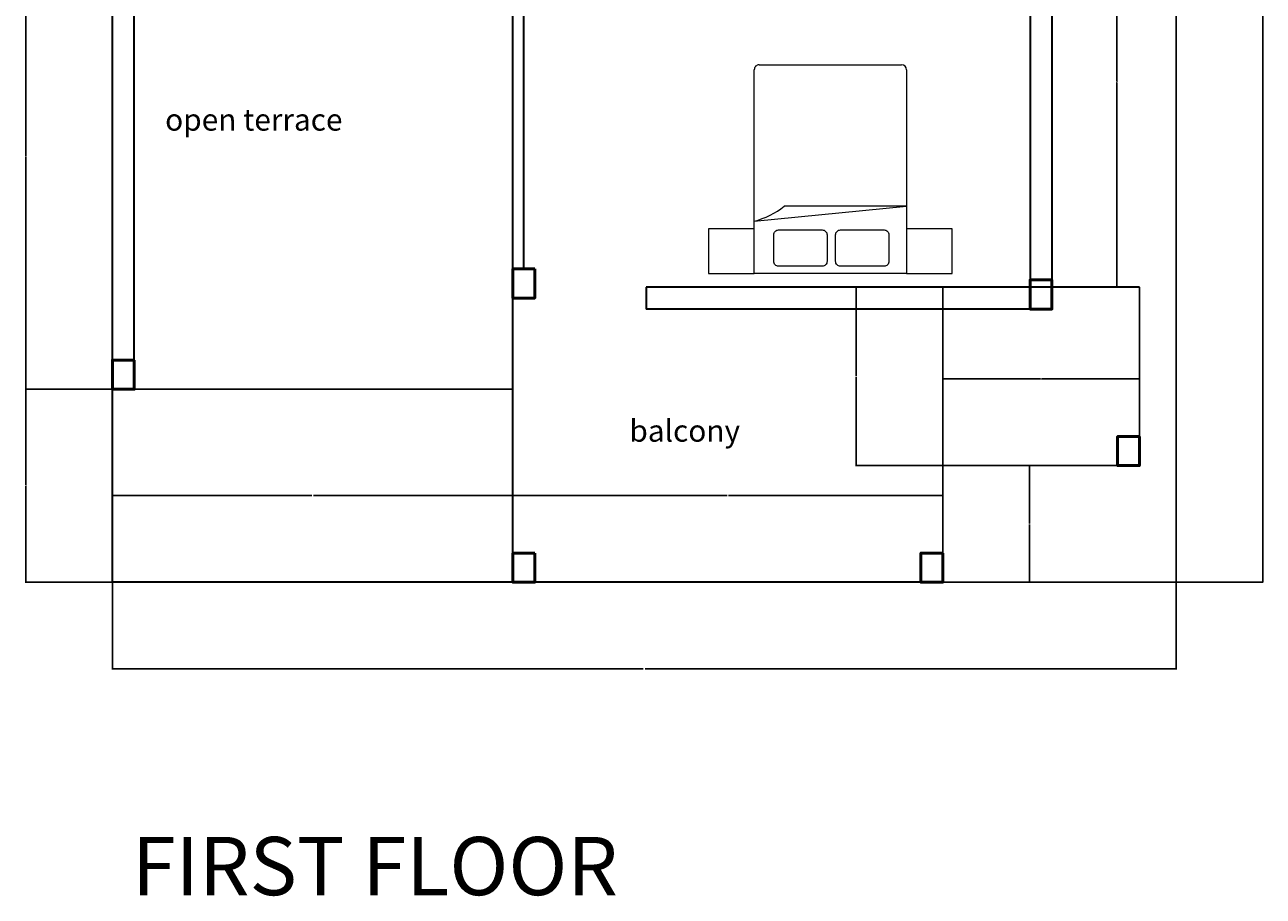
# Model space of a CAD drawing. Units: inches. Extents: x 1748 to 3019, y 1454 to 2188.
# Tile 3 of 4: x 2509 to 3019, y 1459 to 1818. Entities that reach past the tile are written whole.
import ezdxf

# ---------------------------------------------------------------- set-up
doc = ezdxf.new("R2010")
doc.units = ezdxf.units.IN
for name, color, linetype, lineweight in [('A-ANNO-DIMS', 2, 'Continuous', 18), ('A-ANNO-TEXT', 7, 'Continuous', 35), ('A-AREA-IDEN', 134, 'Continuous', 18), ('A-COLS', 120, 'Continuous', 50), ('A-FLOR', 8, 'Continuous', 25), ('A-WALL', 7, 'Continuous', 35), ('bed', 21, 'Continuous', 18)]:
    doc.layers.add(name, color=color, linetype=linetype, lineweight=lineweight)
doc.styles.get("Standard").update_dxf_attribs({"font": 'arial.ttf'})
doc.dimstyles.get("Standard").update_dxf_attribs({"dimtxt": 0.18, "dimasz": 0.18, "dimexe": 0.18, "dimexo": 0.0625, "dimgap": 0.09, "dimtad": 0, "dimtih": 1, "dimtoh": 1, "dimdec": 4, "dimzin": 0, "dimdsep": 46, "dimtxsty": 'Standard', "dimcen": 0.09, "dimadec": 0, "dimazin": 0, "dimtfac": 1, "dimtdec": 4, "dimtofl": 0, "dimtmove": 0, "dimatfit": 3, "dimfxl": 1, "dimtolj": 1, "dimtzin": 0, "dimarcsym": 0})

# ---------------------------------------------------------------- blocks, each defined once
blk = doc.blocks.new('BED-DOUBLE-NIGHTSTANDS')
for p, q in [((0, 81.51), (83.98, 81.51)), ((0, 18.79), (0, 81.51)), ((21.61, 81.51), (27.83, 18.79)), ((85.98, 79.51), (85.98, 20.79)), ((27.83, 18.79), (27.83, 69.19)), ((83.98, 18.79), (0, 18.79))]:
    blk.add_line(p, q)
for points in [[(0, 81.51), (18.52, 81.51), (18.52, 100.3), (0, 100.3)], [(0, 0), (18.52, 0), (18.52, 18.79), (0, 18.79)]]:
    blk.add_lwpolyline(points, close=True)
for points in [[(5.06, 73.49), (16.01, 73.49, -0.414214), (18.01, 71.49), (18.01, 53.51, -0.414214), (16.01, 51.51), (5.06, 51.51, -0.414214), (3.06, 53.51), (3.06, 71.49, -0.414214)], [(5.06, 47.99), (16.01, 47.99, -0.414214), (18.01, 45.99), (18.01, 28.02, -0.414214), (16.01, 26.02), (5.06, 26.02, -0.414214), (3.06, 28.02), (3.06, 45.99, -0.414214)]]:
    blk.add_lwpolyline(points, format="xyb", close=True)
for centre, radius, start, end in [((52.42, 89.31), 31.78, 194.1991, 219.2902), ((83.98, 79.51), 2, 0, 90), ((83.98, 79.51), 2, 0, 90), ((83.98, 20.79), 2, 270, 0)]:
    blk.add_arc(centre, radius, start, end)
blk = doc.blocks.new('COLUMN-9X12')
blk.add_lwpolyline([(9, 12), (9, 0), (0, 0), (0, 12)], close=True)
blk = doc.blocks.new('*D44')
at = {"layer": 'A-ANNO-DIMS', "color": 0, "lineweight": -2, "transparency": 16777216}
for p, q in [((2982.74, 1877), (2982.74, 1552.06)), ((2544.64, 1587.88), (2544.64, 1552.06)), ((2544.82, 1552.24), (2763.31, 1552.24)), ((2982.56, 1552.24), (2764.07, 1552.24))]:
    blk.add_line(p, q, dxfattribs=at)
at = {"layer": 'A-ANNO-DIMS', "color": 0, "transparency": 16777216}
for points in [[(2544.82, 1552.27), (2544.82, 1552.21), (2544.64, 1552.24)], [(2982.56, 1552.27), (2982.56, 1552.21), (2982.74, 1552.24)]]:
    blk.add_solid(points, dxfattribs=at)
at = {"layer": 'Defpoints', "color": 0, "transparency": 16777216}
for p in [(2982.74, 1877.06), (2544.64, 1587.94), (2982.74, 1552.24)]:
    blk.add_point(p, dxfattribs=at)
at = {"layer": 'A-ANNO-DIMS', "color": 0, "transparency": 16777216, "insert": (2763.69, 1552.24), "char_height": 0.18, "attachment_point": 5}
blk.add_mtext('\\A1;438.1', dxfattribs=at)
blk = doc.blocks.new('*D45')
at = {"layer": 'A-ANNO-DIMS', "color": 0, "lineweight": -2, "transparency": 16777216}
for p, q in [((2931.7, 2151.94), (3018.62, 2151.94)), ((3018.44, 2151.76), (3018.44, 1870.12)), ((3018.44, 1588.12), (3018.44, 1869.76)), ((2886.7, 1587.94), (3018.62, 1587.94))]:
    blk.add_line(p, q, dxfattribs=at)
at = {"layer": 'A-ANNO-DIMS', "color": 0, "transparency": 16777216}
for points in [[(3018.41, 2151.76), (3018.47, 2151.76), (3018.44, 2151.94)], [(3018.41, 1588.12), (3018.47, 1588.12), (3018.44, 1587.94)]]:
    blk.add_solid(points, dxfattribs=at)
at = {"layer": 'Defpoints', "color": 0, "transparency": 16777216}
for p in [(2931.64, 2151.94), (3018.44, 2151.94), (2886.64, 1587.94)]:
    blk.add_point(p, dxfattribs=at)
at = {"layer": 'A-ANNO-DIMS', "color": 0, "transparency": 16777216, "insert": (3018.44, 1869.94), "char_height": 0.18, "attachment_point": 5}
blk.add_mtext('\\A1;564', dxfattribs=at)
blk = doc.blocks.new('*D53')
at = {"layer": 'A-ANNO-DIMS', "color": 0, "lineweight": -2, "transparency": 16777216}
for p, q in [((2544.57, 1859.39), (2508.76, 1859.39)), ((2508.94, 1859.21), (2508.94, 1763.6)), ((2508.94, 1667.62), (2508.94, 1763.23)), ((2544.57, 1667.44), (2508.76, 1667.44))]:
    blk.add_line(p, q, dxfattribs=at)
at = {"layer": 'A-ANNO-DIMS', "color": 0, "transparency": 16777216}
for points in [[(2508.91, 1859.21), (2508.97, 1859.21), (2508.94, 1859.39)], [(2508.91, 1667.62), (2508.97, 1667.62), (2508.94, 1667.44)]]:
    blk.add_solid(points, dxfattribs=at)
at = {"layer": 'Defpoints', "color": 0, "transparency": 16777216}
for p in [(2508.94, 1859.39), (2544.64, 1859.39), (2544.64, 1667.44)]:
    blk.add_point(p, dxfattribs=at)
at = {"layer": 'A-ANNO-DIMS', "color": 0, "transparency": 16777216, "insert": (2508.94, 1763.42), "char_height": 0.18, "attachment_point": 5}
blk.add_mtext('\\A1;191.95', dxfattribs=at)
blk = doc.blocks.new('*D54')
at = {"layer": 'A-ANNO-DIMS', "color": 0, "lineweight": -2, "transparency": 16777216}
for p, q in [((2544.57, 1667.44), (2508.76, 1667.44)), ((2508.94, 1667.26), (2508.94, 1627.87)), ((2508.94, 1588.12), (2508.94, 1627.51)), ((2544.57, 1587.94), (2508.76, 1587.94))]:
    blk.add_line(p, q, dxfattribs=at)
at = {"layer": 'A-ANNO-DIMS', "color": 0, "transparency": 16777216}
for points in [[(2508.91, 1667.26), (2508.97, 1667.26), (2508.94, 1667.44)], [(2508.91, 1588.12), (2508.97, 1588.12), (2508.94, 1587.94)]]:
    blk.add_solid(points, dxfattribs=at)
at = {"layer": 'Defpoints', "color": 0, "transparency": 16777216}
for p in [(2508.94, 1667.44), (2544.64, 1667.44), (2544.64, 1587.94)]:
    blk.add_point(p, dxfattribs=at)
at = {"layer": 'A-ANNO-DIMS', "color": 0, "transparency": 16777216, "insert": (2508.94, 1627.69), "char_height": 0.18, "attachment_point": 5}
blk.add_mtext('\\A1;79.5', dxfattribs=at)
blk = doc.blocks.new('*D55')
at = {"layer": 'A-ANNO-DIMS', "color": 0, "lineweight": -2, "transparency": 16777216}
for p, q in [((2922.7, 1878.41), (2958.52, 1878.41)), ((2958.34, 1878.23), (2958.34, 1794.11)), ((2958.34, 1709.62), (2958.34, 1793.74)), ((2922.7, 1709.44), (2958.52, 1709.44))]:
    blk.add_line(p, q, dxfattribs=at)
at = {"layer": 'A-ANNO-DIMS', "color": 0, "transparency": 16777216}
for points in [[(2958.31, 1878.23), (2958.37, 1878.23), (2958.34, 1878.41)], [(2958.31, 1709.62), (2958.37, 1709.62), (2958.34, 1709.44)]]:
    blk.add_solid(points, dxfattribs=at)
at = {"layer": 'Defpoints', "color": 0, "transparency": 16777216}
for p in [(2922.64, 1878.41), (2922.64, 1709.44), (2958.34, 1709.44)]:
    blk.add_point(p, dxfattribs=at)
at = {"layer": 'A-ANNO-DIMS', "color": 0, "transparency": 16777216, "insert": (2958.34, 1793.93), "char_height": 0.18, "attachment_point": 5}
blk.add_mtext('\\A1;168.97', dxfattribs=at)
blk = doc.blocks.new('*D56')
at = {"layer": 'A-ANNO-DIMS', "color": 0, "lineweight": -2, "transparency": 16777216}
for p, q in [((2544.64, 1588), (2544.64, 1623.82)), ((2544.82, 1623.64), (2626.85, 1623.64)), ((2709.46, 1623.64), (2627.42, 1623.64)), ((2709.64, 1588), (2709.64, 1623.82))]:
    blk.add_line(p, q, dxfattribs=at)
at = {"layer": 'A-ANNO-DIMS', "color": 0, "transparency": 16777216}
for points in [[(2544.82, 1623.67), (2544.82, 1623.61), (2544.64, 1623.64)], [(2709.46, 1623.67), (2709.46, 1623.61), (2709.64, 1623.64)]]:
    blk.add_solid(points, dxfattribs=at)
at = {"layer": 'Defpoints', "color": 0, "transparency": 16777216}
for p in [(2709.64, 1623.64), (2544.64, 1587.94), (2709.64, 1587.94)]:
    blk.add_point(p, dxfattribs=at)
at = {"layer": 'A-ANNO-DIMS', "color": 0, "transparency": 16777216, "insert": (2627.14, 1623.64), "char_height": 0.18, "attachment_point": 5}
blk.add_mtext('\\A1;165', dxfattribs=at)
blk = doc.blocks.new('*D57')
at = {"layer": 'A-ANNO-DIMS', "color": 0, "lineweight": -2, "transparency": 16777216}
for p, q in [((2709.64, 1588), (2709.64, 1623.82)), ((2709.82, 1623.64), (2797.85, 1623.64)), ((2886.46, 1623.64), (2798.42, 1623.64)), ((2886.64, 1588), (2886.64, 1623.82))]:
    blk.add_line(p, q, dxfattribs=at)
at = {"layer": 'A-ANNO-DIMS', "color": 0, "transparency": 16777216}
for points in [[(2709.82, 1623.67), (2709.82, 1623.61), (2709.64, 1623.64)], [(2886.46, 1623.67), (2886.46, 1623.61), (2886.64, 1623.64)]]:
    blk.add_solid(points, dxfattribs=at)
at = {"layer": 'Defpoints', "color": 0, "transparency": 16777216}
for p in [(2886.64, 1623.64), (2709.64, 1587.94), (2886.64, 1587.94)]:
    blk.add_point(p, dxfattribs=at)
at = {"layer": 'A-ANNO-DIMS', "color": 0, "transparency": 16777216, "insert": (2798.14, 1623.64), "char_height": 0.18, "attachment_point": 5}
blk.add_mtext('\\A1;177', dxfattribs=at)
blk = doc.blocks.new('*D58')
at = {"layer": 'A-ANNO-DIMS', "color": 0, "lineweight": -2, "transparency": 16777216}
for p, q in [((2886.57, 1709.44), (2850.76, 1709.44)), ((2850.94, 1709.26), (2850.94, 1672.87)), ((2850.94, 1636.12), (2850.94, 1672.51)), ((2886.57, 1635.94), (2850.76, 1635.94))]:
    blk.add_line(p, q, dxfattribs=at)
at = {"layer": 'A-ANNO-DIMS', "color": 0, "transparency": 16777216}
for points in [[(2850.91, 1709.26), (2850.97, 1709.26), (2850.94, 1709.44)], [(2850.91, 1636.12), (2850.97, 1636.12), (2850.94, 1635.94)]]:
    blk.add_solid(points, dxfattribs=at)
at = {"layer": 'Defpoints', "color": 0, "transparency": 16777216}
for p in [(2850.94, 1709.44), (2886.64, 1709.44), (2886.64, 1635.94)]:
    blk.add_point(p, dxfattribs=at)
at = {"layer": 'A-ANNO-DIMS', "color": 0, "transparency": 16777216, "insert": (2850.94, 1672.69), "char_height": 0.18, "attachment_point": 5}
blk.add_mtext('\\A1;73.5', dxfattribs=at)
blk = doc.blocks.new('*D59')
at = {"layer": 'A-ANNO-DIMS', "color": 0, "lineweight": -2, "transparency": 16777216}
for p, q in [((2886.7, 1635.94), (2922.52, 1635.94)), ((2922.34, 1635.76), (2922.34, 1612.12)), ((2922.34, 1588.12), (2922.34, 1611.76)), ((2886.7, 1587.94), (2922.52, 1587.94))]:
    blk.add_line(p, q, dxfattribs=at)
at = {"layer": 'A-ANNO-DIMS', "color": 0, "transparency": 16777216}
for points in [[(2922.31, 1635.76), (2922.37, 1635.76), (2922.34, 1635.94)], [(2922.31, 1588.12), (2922.37, 1588.12), (2922.34, 1587.94)]]:
    blk.add_solid(points, dxfattribs=at)
at = {"layer": 'Defpoints', "color": 0, "transparency": 16777216}
for p in [(2886.64, 1635.94), (2886.64, 1587.94), (2922.34, 1587.94)]:
    blk.add_point(p, dxfattribs=at)
at = {"layer": 'A-ANNO-DIMS', "color": 0, "transparency": 16777216, "insert": (2922.34, 1611.94), "char_height": 0.18, "attachment_point": 5}
blk.add_mtext('\\A1;48', dxfattribs=at)
blk = doc.blocks.new('*D60')
at = {"layer": 'A-ANNO-DIMS', "color": 0, "lineweight": -2, "transparency": 16777216}
for p, q in [((2886.64, 1636), (2886.64, 1671.82)), ((2886.82, 1671.64), (2926.93, 1671.64)), ((2967.46, 1671.64), (2927.34, 1671.64)), ((2967.64, 1636), (2967.64, 1671.82))]:
    blk.add_line(p, q, dxfattribs=at)
at = {"layer": 'A-ANNO-DIMS', "color": 0, "transparency": 16777216}
for points in [[(2886.82, 1671.67), (2886.82, 1671.61), (2886.64, 1671.64)], [(2967.46, 1671.67), (2967.46, 1671.61), (2967.64, 1671.64)]]:
    blk.add_solid(points, dxfattribs=at)
at = {"layer": 'Defpoints', "color": 0, "transparency": 16777216}
for p in [(2967.64, 1671.64), (2886.64, 1635.94), (2967.64, 1635.94)]:
    blk.add_point(p, dxfattribs=at)
at = {"layer": 'A-ANNO-DIMS', "color": 0, "transparency": 16777216, "insert": (2927.14, 1671.64), "char_height": 0.18, "attachment_point": 5}
blk.add_mtext('\\A1;81', dxfattribs=at)

msp = doc.modelspace()

# ---------------------------------------------------------------- linework, layer by layer
at = {"layer": 'A-FLOR'}
for p, q in [((2886.6353, 1644.94), (2886.6353, 1709.44)), ((2967.6353, 1635.94), (2967.6353, 1709.44)), ((2544.6353, 1667.44), (2709.6353, 1667.44)), ((2958.6353, 1644.94), (2958.6353, 1647.94)), ((2886.6353, 1587.94), (2886.6353, 1644.94)), ((2967.6353, 1635.94), (2886.6353, 1635.94))]:
    msp.add_line(p, q, dxfattribs=at)
at = {"layer": 'A-WALL'}
for p, q in [((2922.6353, 2142.94), (2922.6353, 1709.44)), ((2714.1353, 1716.94), (2714.1353, 1863.94)), ((2553.6353, 1667.44), (2553.6353, 1859.44)), ((2709.6353, 1587.94), (2709.6353, 1859.44)), ((2967.6353, 1709.44), (2764.5076, 1709.44)), ((2764.5076, 1709.44), (2764.5076, 1700.44)), ((2931.6353, 1700.44), (2764.5076, 1700.44))]:
    msp.add_line(p, q, dxfattribs=at)
msp.add_lwpolyline([(2886.6353, 1587.94), (2544.6353, 1587.94), (2544.6353, 2151.94), (2931.6353, 2151.94), (2931.6353, 1709.44)], dxfattribs=at)

# ---------------------------------------------------------------- block references
at = {"layer": 'A-COLS'}
for p in [(2709.6349, 1704.94), (2922.6349, 1700.44), (2544.6349, 1667.44), (2958.6349, 1635.94), (2709.6349, 1587.94), (2877.6349, 1587.94)]:
    msp.add_blockref('COLUMN-9X12', p, dxfattribs=at)
at = {"layer": 'bed', "rotation": 89.99999999999962}
msp.add_blockref('BED-DOUBLE-NIGHTSTANDS', (2890.5185, 1715.017), dxfattribs=at)

# ---------------------------------------------------------------- texts
at = {"layer": 'A-ANNO-TEXT', "insert": (2552.6888, 1483.0463), "char_height": 24, "attachment_point": 1}
msp.add_mtext_dynamic_manual_height_columns('FIRST FLOOR', width=613.135788, gutter_width=12.5, heights=[0], dxfattribs=at)
at = {"layer": 'A-AREA-IDEN', "char_height": 9, "attachment_point": 1}
for s, width, insert in [('open terrace', 94.454348, (2566.381, 1782.9213)), ('balcony', 119.179894, (2757.5913, 1654.8119))]:
    msp.add_mtext_dynamic_manual_height_columns(s, width=width, gutter_width=12.5, heights=[0], dxfattribs=dict(at, insert=insert))

# ---------------------------------------------------------------- dimensions: what is measured, and where the dimension line sits
at = {"layer": 'A-ANNO-DIMS'}
for base, p1, p2, angle, override, picture, middle in [((3018.4428, 2151.94), (2886.6353, 1587.94), (2931.6353, 2151.94), 90, {"dimdec": 0, "dimlfac": 1, "dimrnd": 0, "dimzin": 0, "dimdsep": 46, "dimlunit": 2}, '*D45', (3018.4428, 1869.94)), ((2958.3353, 1709.44), (2922.6353, 1878.412), (2922.6353, 1709.44), 270, {"dimdec": 2, "dimlfac": 1, "dimrnd": 0, "dimzin": 0, "dimdsep": 46, "dimlunit": 2}, '*D55', (2958.3353, 1793.926)), ((2508.9353, 1859.3932), (2544.6353, 1667.44), (2544.6353, 1859.3932), 90, {"dimdec": 2, "dimlfac": 1, "dimrnd": 0, "dimzin": 0, "dimdsep": 46, "dimlunit": 2}, '*D53', (2508.9353, 1763.4166)), ((2850.9353, 1709.44), (2886.6353, 1635.94), (2886.6353, 1709.44), 90, {"dimdec": 1, "dimlfac": 1, "dimrnd": 0, "dimzin": 0, "dimdsep": 46, "dimlunit": 2}, '*D58', (2850.9353, 1672.69)), ((2967.6353, 1671.64), (2886.6353, 1635.94), (2967.6353, 1635.94), 0, {"dimdec": 0, "dimlfac": 1, "dimrnd": 0, "dimzin": 0, "dimdsep": 46, "dimlunit": 2}, '*D60', (2927.1353, 1671.64)), ((2508.9353, 1667.44), (2544.6353, 1587.94), (2544.6353, 1667.44), 90, {"dimdec": 1, "dimlfac": 1, "dimrnd": 0, "dimzin": 0, "dimdsep": 46, "dimlunit": 2}, '*D54', (2508.9353, 1627.69)), ((2922.3353, 1587.94), (2886.6353, 1635.94), (2886.6353, 1587.94), 270, {"dimdec": 0, "dimlfac": 1, "dimrnd": 0, "dimzin": 0, "dimdsep": 46, "dimlunit": 2}, '*D59', (2922.3353, 1611.94)), ((2709.6353, 1623.64), (2544.6353, 1587.94), (2709.6353, 1587.94), 0, {"dimdec": 0, "dimlfac": 1, "dimrnd": 0, "dimzin": 0, "dimdsep": 46, "dimlunit": 2}, '*D56', (2627.1353, 1623.64)), ((2886.6353, 1623.64), (2709.6353, 1587.94), (2886.6353, 1587.94), 0, {"dimdec": 0, "dimlfac": 1, "dimrnd": 0, "dimzin": 0, "dimdsep": 46, "dimlunit": 2}, '*D57', (2798.1353, 1623.64))]:
    dim = msp.add_linear_dim(base=base, p1=p1, p2=p2, angle=angle, dimstyle='Standard', override=override, dxfattribs=at)
    dim.commit()
    dim.dimension.update_dxf_attribs({"geometry": picture, "text_midpoint": middle})
dim = msp.add_linear_dim(base=(2982.7428, 1552.24), p1=(2544.6353, 1587.94), p2=(2982.7428, 1877.0584), dimstyle='Standard', override={"dimdec": 1, "dimlfac": 1, "dimrnd": 0, "dimzin": 0, "dimdsep": 46, "dimlunit": 2}, dxfattribs=at)
dim.commit()
dim.dimension.update_dxf_attribs({"geometry": '*D44', "text_midpoint": (2763.689, 1552.24)})

doc.saveas('drawing.dxf')
